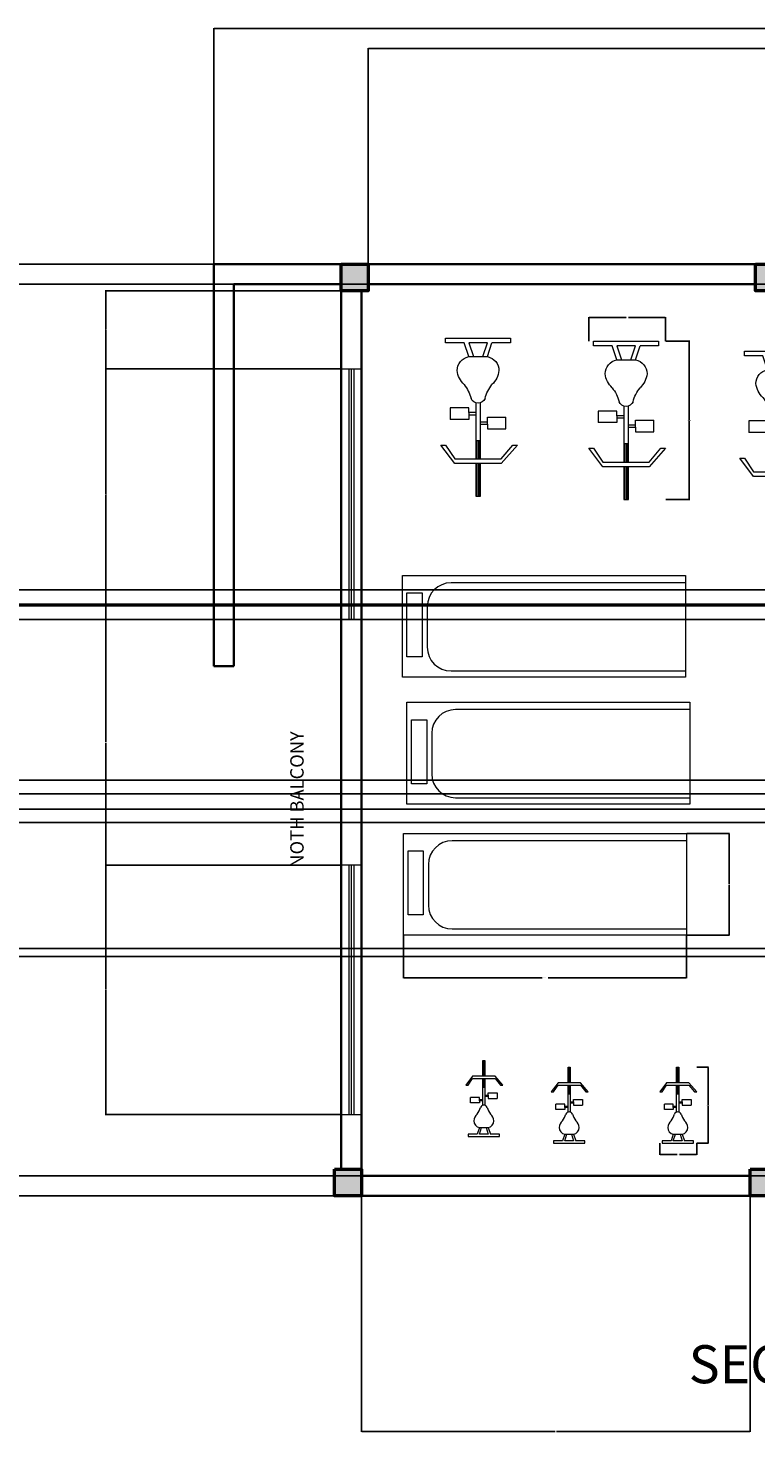
# Model space of a CAD drawing. Units: inches. Extents: x 369 to 4994, y 516 to 1297.
# Tile 7 of 9: x 1910 to 2235, y 516 to 1144. Entities that reach past the tile are written whole.
import ezdxf

# ---------------------------------------------------------------- set-up
doc = ezdxf.new("R2010")
doc.units = ezdxf.units.IN
doc.header["$MEASUREMENT"] = 0
for name, color, linetype, lineweight in [('A-ANNO-DIMS', 2, 'Continuous', 18), ('A-ANNO-TEXT', 7, 'Continuous', 35), ('A-AREA-IDEN', 7, 'Continuous', 18), ('A-COLS', 7, 'Continuous', 50), ('A-EQPM', 9, 'Continuous', 18), ('A-GLAZ', 4, 'Continuous', 18), ('A-WALL', 7, 'Continuous', 35)]:
    doc.layers.add(name, color=color, linetype=linetype, lineweight=lineweight)
doc.layers.add('A-COLS-PATT', color=18, linetype='Continuous', lineweight=13, true_color=0x000000)
doc.styles.get("Standard").update_dxf_attribs({"font": 'arial.ttf'})
doc.dimstyles.get("Standard").update_dxf_attribs({"dimtxt": 0.18, "dimasz": 0.18, "dimexe": 0.18, "dimexo": 0.0625, "dimgap": 0.09, "dimtad": 0, "dimtih": 1, "dimtoh": 1, "dimdec": 4, "dimzin": 0, "dimdsep": 46, "dimtxsty": 'Standard', "dimcen": 0.09, "dimadec": 0, "dimazin": 0, "dimtfac": 1, "dimtdec": 4, "dimtofl": 0, "dimtmove": 0, "dimatfit": 3, "dimfxl": 1, "dimtolj": 1, "dimtzin": 0, "dimarcsym": 0})

# ---------------------------------------------------------------- blocks, each defined once
blk = doc.blocks.new('Exercise Bike')
for p, q in [((-0.75, 10), (-0.75, 17)), ((-0.75, 17), (0.25, 17)), ((-0.5, 17), (-0.5, 9.9929)), ((-0.25, 10), (-0.25, 17)), ((0, 17), (0, 9.9929)), ((0.25, 17), (0.25, 10)), ((-5.25, 10), (-8.25, 6)), ((-0.75, 10), (-5.25, 10)), ((4.75, 10), (-0.75, 10)), ((8.25, 6), (4.75, 10)), ((-7.25, 6), (-5.25, 9)), ((-5.25, 9), (4.75, 9)), ((-0.75, 5), (-0.75, 9)), ((-0.5, 8.9396), (-0.5, 5)), ((-0.25, 5), (-0.25, 9)), ((0, 8.9396), (0, 5)), ((0.25, 9), (0.25, 5)), ((4.75, 9), (7.25, 6)), ((-8.25, 6), (-7.25, 6)), ((-0.75, -3.0635), (-0.75, 5)), ((-0.75, 5), (0.25, 5)), ((0.25, 5), (0.25, -3.0635)), ((7.25, 6), (8.25, 6)), ((-6.25, -2), (-6.25, 0.5)), ((-2.25, 0.5), (-6.25, 0.5)), ((-2.25, -0.5), (-2.25, 0.5)), ((0.25, 1.5), (1.75, 1.5)), ((0.25, 1), (1.75, 1)), ((1.75, 2.5), (5.75, 2.5)), ((1.75, 1.5), (1.75, 2.5)), ((1.75, 1.5), (1.75, 0)), ((1.75, 0), (5.75, 0)), ((5.75, 2.5), (5.75, 0)), ((-2.25, -2), (-6.25, -2)), ((-2.25, -0.5), (-0.75, -0.5)), ((-2.25, -1), (-2.25, -0.5)), ((-2.25, -1), (-2.25, -2)), ((-0.75, -1), (-2.25, -1)), ((-2.25, -13), (-3.25, -16)), ((-2.25, -16), (-1.25, -13)), ((-2.25, -13), (1.75, -13)), ((0.75, -13), (1.75, -16)), ((1.75, -13), (2.75, -16)), ((-7.25, -16), (-7.25, -17)), ((-4.75, -16), (-7.25, -16)), ((-7.25, -17), (6.75, -17)), ((-3.25, -16), (-4.75, -16)), ((1.75, -16), (-2.25, -16)), ((6.75, -16), (2.75, -16)), ((6.75, -17), (6.75, -16))]:
    blk.add_line(p, q)
for centre, radius, start, end in [((-0.25, -4.625), 1.625, 22.61987, 157.3801), ((-9.6692, -1.9154), 8.1889, 321.6175, 345.2525), ((9.1691, -1.9154), 8.1889, 194.7476, 218.3825), ((0.1685, -10.5843), 4.9531, 133.6443, 173.2256), ((-0.6686, -10.5843), 4.9531, 6.774486, 46.35562), ((-1.7006, -10.0005), 3.0494, 179.9906, 259.6205), ((1.2006, -10.0005), 3.0494, 280.3795, 0.009389)]:
    blk.add_arc(centre, radius, start, end)
blk = doc.blocks.new('GYM-TREADMILL')
for p, q in [((126.66, 42.28), (21.77, 42.28)), ((11.14, 31.65), (11.14, 13.47)), ((21.77, 2.84), (126.66, 2.84))]:
    blk.add_line(p, q)
for points in [[(0, 45.56), (126.66, 45.56), (126.66, 0), (0, 0)], [(2.08, 37.74), (8.86, 37.74), (8.86, 9.1), (2.08, 9.1)]]:
    blk.add_lwpolyline(points, close=True)
for centre, start, end in [((21.77, 31.65), 90, 180), ((21.77, 13.47), 180, 270)]:
    blk.add_arc(centre, 10.63, start, end)
blk = doc.blocks.new('BALCONY-EDGE')
for p, q in [((57, 180), (0, 180)), ((0, 180), (0, 0)), ((9, 171), (9, 0)), ((57, 171), (9, 171)), ((9, 0), (0, 0))]:
    blk.add_line(p, q)
blk = doc.blocks.new('*D31')
at = {"layer": 'A-ANNO-DIMS', "color": 0, "lineweight": -2, "transparency": 16777216}
for p, q in [((2209.04, 679.42), (2214.25, 679.42)), ((2214.07, 679.24), (2214.07, 662.61)), ((2214.07, 645.6), (2214.07, 662.24)), ((2209.04, 645.42), (2214.25, 645.42))]:
    blk.add_line(p, q, dxfattribs=at)
at = {"layer": 'A-ANNO-DIMS', "color": 0, "transparency": 16777216}
for points in [[(2214.04, 679.24), (2214.1, 679.24), (2214.07, 679.42)], [(2214.04, 645.6), (2214.1, 645.6), (2214.07, 645.42)]]:
    blk.add_solid(points, dxfattribs=at)
at = {"layer": 'Defpoints', "color": 0, "transparency": 16777216}
for p in [(2208.97, 679.42), (2214.07, 679.42), (2208.97, 645.42)]:
    blk.add_point(p, dxfattribs=at)
at = {"layer": 'A-ANNO-DIMS', "color": 0, "transparency": 16777216, "insert": (2214.07, 662.42), "char_height": 0.18, "attachment_point": 5}
blk.add_mtext('\\A1;BIKE 34 TYP.', dxfattribs=at)
blk = doc.blocks.new('*D32')
at = {"layer": 'A-ANNO-DIMS', "color": 0, "lineweight": -2, "transparency": 16777216}
for p, q in [((2192.47, 645.36), (2192.47, 640.14)), ((2208.97, 645.36), (2208.97, 640.14)), ((2192.65, 640.32), (2200.21, 640.32)), ((2208.79, 640.32), (2201.24, 640.32))]:
    blk.add_line(p, q, dxfattribs=at)
at = {"layer": 'A-ANNO-DIMS', "color": 0, "transparency": 16777216}
for points in [[(2192.65, 640.35), (2192.65, 640.29), (2192.47, 640.32)], [(2208.79, 640.35), (2208.79, 640.29), (2208.97, 640.32)]]:
    blk.add_solid(points, dxfattribs=at)
at = {"layer": 'Defpoints', "color": 0, "transparency": 16777216}
for p in [(2192.47, 645.42), (2208.97, 645.42), (2208.97, 640.32)]:
    blk.add_point(p, dxfattribs=at)
at = {"layer": 'A-ANNO-DIMS', "color": 0, "transparency": 16777216, "insert": (2200.72, 640.32), "char_height": 0.18, "attachment_point": 5}
blk.add_mtext('\\A1;17 TYP.', dxfattribs=at)
blk = doc.blocks.new('*D33')
at = {"layer": 'A-ANNO-DIMS', "color": 0, "lineweight": -2, "transparency": 16777216}
for p, q in [((2195.09, 1004.23), (2205.82, 1004.23)), ((2205.64, 1004.05), (2205.64, 969.04)), ((2205.64, 933.67), (2205.64, 968.68)), ((2195.09, 933.49), (2205.82, 933.49))]:
    blk.add_line(p, q, dxfattribs=at)
at = {"layer": 'A-ANNO-DIMS', "color": 0, "transparency": 16777216}
for points in [[(2205.61, 1004.05), (2205.67, 1004.05), (2205.64, 1004.23)], [(2205.61, 933.67), (2205.67, 933.67), (2205.64, 933.49)]]:
    blk.add_solid(points, dxfattribs=at)
at = {"layer": 'Defpoints', "color": 0, "transparency": 16777216}
for p in [(2195.03, 1004.23), (2195.03, 933.49), (2205.64, 933.49)]:
    blk.add_point(p, dxfattribs=at)
at = {"layer": 'A-ANNO-DIMS', "color": 0, "transparency": 16777216, "insert": (2205.64, 968.86), "char_height": 0.18, "attachment_point": 5}
blk.add_mtext('\\A1;BIKE 71 TYP.', dxfattribs=at)
blk = doc.blocks.new('*D34')
at = {"layer": 'A-ANNO-DIMS', "color": 0, "lineweight": -2, "transparency": 16777216}
for p, q in [((2160.71, 1004.29), (2160.71, 1015.02)), ((2160.89, 1014.84), (2177.34, 1014.84)), ((2194.85, 1014.84), (2178.4, 1014.84)), ((2195.03, 1004.29), (2195.03, 1015.02))]:
    blk.add_line(p, q, dxfattribs=at)
at = {"layer": 'A-ANNO-DIMS', "color": 0, "transparency": 16777216}
for points in [[(2160.89, 1014.87), (2160.89, 1014.81), (2160.71, 1014.84)], [(2194.85, 1014.87), (2194.85, 1014.81), (2195.03, 1014.84)]]:
    blk.add_solid(points, dxfattribs=at)
at = {"layer": 'Defpoints', "color": 0, "transparency": 16777216}
for p in [(2195.03, 1014.84), (2160.71, 1004.23), (2195.03, 1004.23)]:
    blk.add_point(p, dxfattribs=at)
at = {"layer": 'A-ANNO-DIMS', "color": 0, "transparency": 16777216, "insert": (2177.87, 1014.84), "char_height": 0.18, "attachment_point": 5}
blk.add_mtext('\\A1;34 TYP.', dxfattribs=at)
blk = doc.blocks.new('*D37')
at = {"layer": 'A-ANNO-DIMS', "color": 0, "lineweight": -2, "transparency": 16777216}
for p, q in [((2077.76, 738.39), (2077.76, 719.27)), ((2204.43, 738.39), (2204.43, 719.27)), ((2077.94, 719.45), (2139.75, 719.45)), ((2204.25, 719.45), (2142.44, 719.45))]:
    blk.add_line(p, q, dxfattribs=at)
at = {"layer": 'A-ANNO-DIMS', "color": 0, "transparency": 16777216}
for points in [[(2077.94, 719.48), (2077.94, 719.42), (2077.76, 719.45)], [(2204.25, 719.48), (2204.25, 719.42), (2204.43, 719.45)]]:
    blk.add_solid(points, dxfattribs=at)
at = {"layer": 'Defpoints', "color": 0, "transparency": 16777216}
for p in [(2077.76, 738.45), (2204.43, 738.45), (2204.43, 719.45)]:
    blk.add_point(p, dxfattribs=at)
at = {"layer": 'A-ANNO-DIMS', "color": 0, "transparency": 16777216, "insert": (2141.1, 719.45), "char_height": 0.18, "attachment_point": 5}
blk.add_mtext('\\A1;TREADMILL 127 TYP.', dxfattribs=at)
blk = doc.blocks.new('*D38')
at = {"layer": 'A-ANNO-DIMS', "color": 0, "lineweight": -2, "transparency": 16777216}
for p, q in [((2204.49, 784.01), (2223.6, 784.01)), ((2223.42, 783.83), (2223.42, 761.41)), ((2223.42, 738.63), (2223.42, 761.05)), ((2204.49, 738.45), (2223.6, 738.45))]:
    blk.add_line(p, q, dxfattribs=at)
at = {"layer": 'A-ANNO-DIMS', "color": 0, "transparency": 16777216}
for points in [[(2223.39, 783.83), (2223.45, 783.83), (2223.42, 784.01)], [(2223.39, 738.63), (2223.45, 738.63), (2223.42, 738.45)]]:
    blk.add_solid(points, dxfattribs=at)
at = {"layer": 'Defpoints', "color": 0, "transparency": 16777216}
for p in [(2204.43, 784.01), (2223.42, 784.01), (2204.43, 738.45)]:
    blk.add_point(p, dxfattribs=at)
at = {"layer": 'A-ANNO-DIMS', "color": 0, "transparency": 16777216, "insert": (2223.42, 761.23), "char_height": 0.18, "attachment_point": 5}
blk.add_mtext('\\A1;46 TYP.', dxfattribs=at)
blk = doc.blocks.new('*D46')
at = {"layer": 'A-ANNO-DIMS', "color": 0, "lineweight": -2, "transparency": 16777216}
for p, q in [((978.32, 1029.79), (2671.51, 1029.79)), ((2671.33, 1029.61), (2671.33, 957.97)), ((2671.33, 885.97), (2671.33, 957.61)), ((1038.32, 885.79), (2671.51, 885.79))]:
    blk.add_line(p, q, dxfattribs=at)
at = {"layer": 'A-ANNO-DIMS', "color": 0, "transparency": 16777216}
for points in [[(2671.3, 1029.61), (2671.36, 1029.61), (2671.33, 1029.79)], [(2671.3, 885.97), (2671.36, 885.97), (2671.33, 885.79)]]:
    blk.add_solid(points, dxfattribs=at)
at = {"layer": 'Defpoints', "color": 0, "transparency": 16777216}
for p in [(978.26, 1029.79), (2671.33, 1029.79), (1038.26, 885.79)]:
    blk.add_point(p, dxfattribs=at)
at = {"layer": 'A-ANNO-DIMS', "color": 0, "transparency": 16777216, "insert": (2671.33, 957.79), "char_height": 0.18, "attachment_point": 5}
blk.add_mtext('\\A1;144', dxfattribs=at)
blk = doc.blocks.new('*D47')
at = {"layer": 'A-ANNO-DIMS', "color": 0, "lineweight": -2, "transparency": 16777216}
for p, q in [((1038.32, 879.79), (2671.51, 879.79)), ((2671.33, 879.61), (2671.33, 837.52)), ((2671.33, 795.07), (2671.33, 837.16)), ((1035.32, 794.89), (2671.51, 794.89))]:
    blk.add_line(p, q, dxfattribs=at)
at = {"layer": 'A-ANNO-DIMS', "color": 0, "transparency": 16777216}
for points in [[(2671.3, 879.61), (2671.36, 879.61), (2671.33, 879.79)], [(2671.3, 795.07), (2671.36, 795.07), (2671.33, 794.89)]]:
    blk.add_solid(points, dxfattribs=at)
at = {"layer": 'Defpoints', "color": 0, "transparency": 16777216}
for p in [(1038.26, 879.79), (2671.33, 879.79), (1035.26, 794.89)]:
    blk.add_point(p, dxfattribs=at)
at = {"layer": 'A-ANNO-DIMS', "color": 0, "transparency": 16777216, "insert": (2671.33, 837.34), "char_height": 0.18, "attachment_point": 5}
blk.add_mtext('\\A1;84.9', dxfattribs=at)
blk = doc.blocks.new('*D52')
at = {"layer": 'A-ANNO-DIMS', "color": 0, "lineweight": -2, "transparency": 16777216}
for p, q in [((942.32, 788.89), (2671.51, 788.89)), ((2671.33, 788.71), (2671.33, 710.02)), ((2671.33, 630.97), (2671.33, 709.66)), ((1035.32, 630.79), (2671.51, 630.79))]:
    blk.add_line(p, q, dxfattribs=at)
at = {"layer": 'A-ANNO-DIMS', "color": 0, "transparency": 16777216}
for points in [[(2671.3, 788.71), (2671.36, 788.71), (2671.33, 788.89)], [(2671.3, 630.97), (2671.36, 630.97), (2671.33, 630.79)]]:
    blk.add_solid(points, dxfattribs=at)
at = {"layer": 'Defpoints', "color": 0, "transparency": 16777216}
for p in [(942.26, 788.89), (2671.33, 788.89), (1035.26, 630.79)]:
    blk.add_point(p, dxfattribs=at)
at = {"layer": 'A-ANNO-DIMS', "color": 0, "transparency": 16777216, "insert": (2671.33, 709.84), "char_height": 0.18, "attachment_point": 5}
blk.add_mtext('\\A1;158.1', dxfattribs=at)
blk = doc.blocks.new('*D79')
at = {"layer": 'A-ANNO-DIMS', "color": 0, "lineweight": -2, "transparency": 16777216}
for p, q in [((1769.44, 1029.79), (2671.51, 1029.79)), ((2671.33, 1029.61), (2671.33, 961.56)), ((2671.33, 893.15), (2671.33, 961.2)), ((1772.44, 892.97), (2671.51, 892.97))]:
    blk.add_line(p, q, dxfattribs=at)
at = {"layer": 'A-ANNO-DIMS', "color": 0, "transparency": 16777216}
for points in [[(2671.3, 1029.61), (2671.36, 1029.61), (2671.33, 1029.79)], [(2671.3, 893.15), (2671.36, 893.15), (2671.33, 892.97)]]:
    blk.add_solid(points, dxfattribs=at)
at = {"layer": 'Defpoints', "color": 0, "transparency": 16777216}
for p in [(1769.37, 1029.79), (2671.33, 1029.79), (1772.37, 892.97)]:
    blk.add_point(p, dxfattribs=at)
at = {"layer": 'A-ANNO-DIMS', "color": 0, "transparency": 16777216, "insert": (2671.33, 961.38), "char_height": 0.18, "attachment_point": 5}
blk.add_mtext('\\A1;136.82', dxfattribs=at)
blk = doc.blocks.new('*D80')
at = {"layer": 'A-ANNO-DIMS', "color": 0, "lineweight": -2, "transparency": 16777216}
for p, q in [((1772.44, 886.6), (2671.51, 886.6)), ((2671.33, 886.42), (2671.33, 847.38)), ((2671.33, 807.97), (2671.33, 847.01)), ((1772.44, 807.79), (2671.51, 807.79))]:
    blk.add_line(p, q, dxfattribs=at)
at = {"layer": 'A-ANNO-DIMS', "color": 0, "transparency": 16777216}
for points in [[(2671.3, 886.42), (2671.36, 886.42), (2671.33, 886.6)], [(2671.3, 807.97), (2671.36, 807.97), (2671.33, 807.79)]]:
    blk.add_solid(points, dxfattribs=at)
at = {"layer": 'Defpoints', "color": 0, "transparency": 16777216}
for p in [(1772.37, 886.6), (2671.33, 886.6), (1772.37, 807.79)]:
    blk.add_point(p, dxfattribs=at)
at = {"layer": 'A-ANNO-DIMS', "color": 0, "transparency": 16777216, "insert": (2671.33, 847.19), "char_height": 0.18, "attachment_point": 5}
blk.add_mtext('\\A1;78.81', dxfattribs=at)
blk = doc.blocks.new('*D85')
at = {"layer": 'A-ANNO-DIMS', "color": 0, "lineweight": -2, "transparency": 16777216}
for p, q in [((1772.44, 801.79), (2671.51, 801.79)), ((2671.33, 801.61), (2671.33, 767.36)), ((2671.33, 732.75), (2671.33, 767)), ((1772.44, 732.57), (2671.51, 732.57))]:
    blk.add_line(p, q, dxfattribs=at)
at = {"layer": 'A-ANNO-DIMS', "color": 0, "transparency": 16777216}
for points in [[(2671.3, 801.61), (2671.36, 801.61), (2671.33, 801.79)], [(2671.3, 732.75), (2671.36, 732.75), (2671.33, 732.57)]]:
    blk.add_solid(points, dxfattribs=at)
at = {"layer": 'Defpoints', "color": 0, "transparency": 16777216}
for p in [(1772.37, 801.79), (2671.33, 801.79), (1772.37, 732.57)]:
    blk.add_point(p, dxfattribs=at)
at = {"layer": 'A-ANNO-DIMS', "color": 0, "transparency": 16777216, "insert": (2671.33, 767.18), "char_height": 0.18, "attachment_point": 5}
blk.add_mtext('\\A1;69.22', dxfattribs=at)
blk = doc.blocks.new('*D86')
at = {"layer": 'A-ANNO-DIMS', "color": 0, "lineweight": -2, "transparency": 16777216}
for p, q in [((1772.44, 728.97), (2671.51, 728.97)), ((2671.33, 728.79), (2671.33, 680.06)), ((2671.33, 630.97), (2671.33, 679.7)), ((1769.44, 630.79), (2671.51, 630.79))]:
    blk.add_line(p, q, dxfattribs=at)
at = {"layer": 'A-ANNO-DIMS', "color": 0, "transparency": 16777216}
for points in [[(2671.3, 728.79), (2671.36, 728.79), (2671.33, 728.97)], [(2671.3, 630.97), (2671.36, 630.97), (2671.33, 630.79)]]:
    blk.add_solid(points, dxfattribs=at)
at = {"layer": 'Defpoints', "color": 0, "transparency": 16777216}
for p in [(1772.37, 728.97), (2671.33, 728.97), (1769.37, 630.79)]:
    blk.add_point(p, dxfattribs=at)
at = {"layer": 'A-ANNO-DIMS', "color": 0, "transparency": 16777216, "insert": (2671.33, 679.88), "char_height": 0.18, "attachment_point": 5}
blk.add_mtext('\\A1;98.18', dxfattribs=at)
blk = doc.blocks.new('*D97')
at = {"layer": 'A-ANNO-DIMS', "color": 0, "lineweight": -2, "transparency": 16777216}
for p, q in [((1992.93, 1038.85), (1992.93, 1144.37)), ((1993.11, 1144.19), (2279.14, 1144.19)), ((2565.75, 1144.19), (2279.72, 1144.19)), ((2565.93, 1038.85), (2565.93, 1144.37))]:
    blk.add_line(p, q, dxfattribs=at)
at = {"layer": 'A-ANNO-DIMS', "color": 0, "transparency": 16777216}
for points in [[(1993.11, 1144.22), (1993.11, 1144.16), (1992.93, 1144.19)], [(2565.75, 1144.22), (2565.75, 1144.16), (2565.93, 1144.19)]]:
    blk.add_solid(points, dxfattribs=at)
at = {"layer": 'Defpoints', "color": 0, "transparency": 16777216}
for p in [(2565.93, 1144.19), (1992.93, 1038.79), (2565.93, 1038.79)]:
    blk.add_point(p, dxfattribs=at)
at = {"layer": 'A-ANNO-DIMS', "color": 0, "transparency": 16777216, "insert": (2279.43, 1144.19), "char_height": 0.18, "attachment_point": 5}
blk.add_mtext('\\A1;573', dxfattribs=at)
blk = doc.blocks.new('*D98')
at = {"layer": 'A-ANNO-DIMS', "color": 0, "lineweight": -2, "transparency": 16777216}
for p, q in [((1992.86, 1038.79), (368.68, 1038.79)), ((368.86, 1038.61), (368.86, 830.47)), ((368.86, 621.97), (368.86, 830.11)), ((2046.86, 621.79), (368.68, 621.79))]:
    blk.add_line(p, q, dxfattribs=at)
at = {"layer": 'A-ANNO-DIMS', "color": 0, "transparency": 16777216}
for points in [[(368.83, 1038.61), (368.89, 1038.61), (368.86, 1038.79)], [(368.83, 621.97), (368.89, 621.97), (368.86, 621.79)]]:
    blk.add_solid(points, dxfattribs=at)
at = {"layer": 'Defpoints', "color": 0, "transparency": 16777216}
for p in [(368.86, 1038.79), (1992.93, 1038.79), (2046.93, 621.79)]:
    blk.add_point(p, dxfattribs=at)
at = {"layer": 'A-ANNO-DIMS', "color": 0, "transparency": 16777216, "insert": (368.86, 830.29), "char_height": 0.18, "attachment_point": 5}
blk.add_mtext('\\A1;417', dxfattribs=at)
blk = doc.blocks.new('*D99')
at = {"layer": 'A-ANNO-DIMS', "color": 0, "lineweight": -2, "transparency": 16777216}
for p, q in [((2061.93, 1029.85), (2061.93, 1135.37)), ((2062.11, 1135.19), (2241.64, 1135.19)), ((2421.75, 1135.19), (2242.22, 1135.19)), ((2421.93, 1029.85), (2421.93, 1135.37))]:
    blk.add_line(p, q, dxfattribs=at)
at = {"layer": 'A-ANNO-DIMS', "color": 0, "transparency": 16777216}
for points in [[(2062.11, 1135.22), (2062.11, 1135.16), (2061.93, 1135.19)], [(2421.75, 1135.22), (2421.75, 1135.16), (2421.93, 1135.19)]]:
    blk.add_solid(points, dxfattribs=at)
at = {"layer": 'Defpoints', "color": 0, "transparency": 16777216}
for p in [(2421.93, 1135.19), (2061.93, 1029.79), (2421.93, 1029.79)]:
    blk.add_point(p, dxfattribs=at)
at = {"layer": 'A-ANNO-DIMS', "color": 0, "transparency": 16777216, "insert": (2241.93, 1135.19), "char_height": 0.18, "attachment_point": 5}
blk.add_mtext('\\A1;360', dxfattribs=at)
blk = doc.blocks.new('*D108')
at = {"layer": 'A-ANNO-DIMS', "color": 0, "lineweight": -2, "transparency": 16777216}
for p, q in [((2058.93, 630.73), (2058.93, 516.21)), ((2232.93, 630.73), (2232.93, 516.21)), ((2059.11, 516.39), (2145.65, 516.39)), ((2232.75, 516.39), (2146.21, 516.39))]:
    blk.add_line(p, q, dxfattribs=at)
at = {"layer": 'A-ANNO-DIMS', "color": 0, "transparency": 16777216}
for points in [[(2059.11, 516.42), (2059.11, 516.36), (2058.93, 516.39)], [(2232.75, 516.42), (2232.75, 516.36), (2232.93, 516.39)]]:
    blk.add_solid(points, dxfattribs=at)
at = {"layer": 'Defpoints', "color": 0, "transparency": 16777216}
for p in [(2058.93, 630.79), (2232.93, 630.79), (2232.93, 516.39)]:
    blk.add_point(p, dxfattribs=at)
at = {"layer": 'A-ANNO-DIMS', "color": 0, "transparency": 16777216, "insert": (2145.93, 516.39), "char_height": 0.18, "attachment_point": 5}
blk.add_mtext('\\A1;174', dxfattribs=at)
blk = doc.blocks.new('*D112')
at = {"layer": 'A-ANNO-DIMS', "color": 0, "lineweight": -2, "transparency": 16777216}
for p, q in [((2049.86, 1026.79), (1944.35, 1026.79)), ((1944.53, 1026.61), (1944.53, 1009.52)), ((1944.53, 992.06), (1944.53, 1009.15)), ((2049.86, 991.88), (1944.35, 991.88))]:
    blk.add_line(p, q, dxfattribs=at)
at = {"layer": 'A-ANNO-DIMS', "color": 0, "transparency": 16777216}
for points in [[(1944.5, 1026.61), (1944.56, 1026.61), (1944.53, 1026.79)], [(1944.5, 992.06), (1944.56, 992.06), (1944.53, 991.88)]]:
    blk.add_solid(points, dxfattribs=at)
at = {"layer": 'Defpoints', "color": 0, "transparency": 16777216}
for p in [(1944.53, 1026.79), (2049.93, 1026.79), (2049.93, 991.88)]:
    blk.add_point(p, dxfattribs=at)
at = {"layer": 'A-ANNO-DIMS', "color": 0, "transparency": 16777216, "insert": (1944.53, 1009.33), "char_height": 0.18, "attachment_point": 5}
blk.add_mtext('\\A1;34.91', dxfattribs=at)
blk = doc.blocks.new('*D113')
at = {"layer": 'A-ANNO-DIMS', "color": 0, "lineweight": -2, "transparency": 16777216}
for p, q in [((2049.86, 991.88), (1944.35, 991.88)), ((1944.53, 991.7), (1944.53, 936.02)), ((1944.53, 879.97), (1944.53, 935.65)), ((2049.86, 879.79), (1944.35, 879.79))]:
    blk.add_line(p, q, dxfattribs=at)
at = {"layer": 'A-ANNO-DIMS', "color": 0, "transparency": 16777216}
for points in [[(1944.5, 991.7), (1944.56, 991.7), (1944.53, 991.88)], [(1944.5, 879.97), (1944.56, 879.97), (1944.53, 879.79)]]:
    blk.add_solid(points, dxfattribs=at)
at = {"layer": 'Defpoints', "color": 0, "transparency": 16777216}
for p in [(1944.53, 991.88), (2049.93, 991.88), (2049.93, 879.79)]:
    blk.add_point(p, dxfattribs=at)
at = {"layer": 'A-ANNO-DIMS', "color": 0, "transparency": 16777216, "insert": (1944.53, 935.83), "char_height": 0.18, "attachment_point": 5}
blk.add_mtext('\\A1;112.09', dxfattribs=at)
blk = doc.blocks.new('*D114')
at = {"layer": 'A-ANNO-DIMS', "color": 0, "lineweight": -2, "transparency": 16777216}
for p, q in [((2049.86, 879.79), (1944.35, 879.79)), ((1944.53, 879.61), (1944.53, 824.97)), ((1944.53, 769.97), (1944.53, 824.61)), ((2049.86, 769.79), (1944.35, 769.79))]:
    blk.add_line(p, q, dxfattribs=at)
at = {"layer": 'A-ANNO-DIMS', "color": 0, "transparency": 16777216}
for points in [[(1944.5, 879.61), (1944.56, 879.61), (1944.53, 879.79)], [(1944.5, 769.97), (1944.56, 769.97), (1944.53, 769.79)]]:
    blk.add_solid(points, dxfattribs=at)
at = {"layer": 'Defpoints', "color": 0, "transparency": 16777216}
for p in [(1944.53, 879.79), (2049.93, 879.79), (2049.93, 769.79)]:
    blk.add_point(p, dxfattribs=at)
at = {"layer": 'A-ANNO-DIMS', "color": 0, "transparency": 16777216, "insert": (1944.53, 824.79), "char_height": 0.18, "attachment_point": 5}
blk.add_mtext('\\A1;110', dxfattribs=at)
blk = doc.blocks.new('*D115')
at = {"layer": 'A-ANNO-DIMS', "color": 0, "lineweight": -2, "transparency": 16777216}
for p, q in [((2049.86, 769.79), (1944.35, 769.79)), ((1944.53, 769.61), (1944.53, 714.2)), ((1944.53, 658.42), (1944.53, 713.84)), ((2049.86, 658.24), (1944.35, 658.24))]:
    blk.add_line(p, q, dxfattribs=at)
at = {"layer": 'A-ANNO-DIMS', "color": 0, "transparency": 16777216}
for points in [[(1944.5, 769.61), (1944.56, 769.61), (1944.53, 769.79)], [(1944.5, 658.42), (1944.56, 658.42), (1944.53, 658.24)]]:
    blk.add_solid(points, dxfattribs=at)
at = {"layer": 'Defpoints', "color": 0, "transparency": 16777216}
for p in [(1944.53, 769.79), (2049.93, 769.79), (2049.93, 658.24)]:
    blk.add_point(p, dxfattribs=at)
at = {"layer": 'A-ANNO-DIMS', "color": 0, "transparency": 16777216, "insert": (1944.53, 714.02), "char_height": 0.18, "attachment_point": 5}
blk.add_mtext('\\A1;111.55', dxfattribs=at)

msp = doc.modelspace()

# ---------------------------------------------------------------- hatches: boundary and pattern name
at = {"layer": 'A-COLS-PATT'}
h = msp.add_hatch(color=256, dxfattribs=at)
h.dxf.hatch_style = 1
h.paths.add_polyline_path([(540.2581, 633.7894), (528.2581, 633.7894), (528.2581, 621.7894), (540.2581, 621.7894)])
h.paths.add_polyline_path([(726.2581, 633.7894), (714.2581, 633.7894), (714.2581, 621.7894), (726.2581, 621.7894)])
h.paths.add_polyline_path([(918.2581, 633.7894), (906.2581, 633.7894), (906.2581, 621.7894), (918.2581, 621.7894)])
h.paths.add_polyline_path([(1047.2581, 633.7894), (1035.2581, 633.7894), (1035.2581, 621.7894), (1047.2581, 621.7894)])
h.paths.add_polyline_path([(1047.2581, 798.6977), (1035.2581, 798.6977), (1035.2581, 786.6977), (1047.2581, 786.6977)])
h.paths.add_polyline_path([(918.2581, 795.7894), (906.2581, 795.7894), (906.2581, 783.7894), (918.2581, 783.7894)])
h.paths.add_polyline_path([(726.2581, 795.7894), (714.2581, 795.7894), (714.2581, 783.7894), (726.2581, 783.7894)])
h.paths.add_polyline_path([(1047.2581, 1038.7894), (1035.2581, 1038.7894), (1035.2581, 1026.7894), (1047.2581, 1026.7894)])
h.paths.add_polyline_path([(855.044, 1038.7894), (843.044, 1038.7894), (843.044, 1026.7894), (855.044, 1026.7894)])
h.paths.add_polyline_path([(728.5536, 1038.7894), (716.5536, 1038.7894), (716.5536, 1026.7894), (728.5536, 1026.7894)])
h.paths.add_polyline_path([(543.2581, 1038.7894), (531.2581, 1038.7894), (531.2581, 1026.7894), (543.2581, 1026.7894)])
h.paths.add_polyline_path([(543.2581, 792.9013), (531.2581, 792.9013), (531.2581, 780.9013), (543.2581, 780.9013), (543.2581, 783.7894)])
h.paths.add_polyline_path([(1274.3738, 633.7894), (1262.3738, 633.7894), (1262.3738, 621.7894), (1274.3738, 621.7894)])
h.paths.add_polyline_path([(1460.3738, 633.7894), (1448.3738, 633.7894), (1448.3738, 621.7894), (1460.3738, 621.7894)])
h.paths.add_polyline_path([(1652.3738, 633.7894), (1640.3738, 633.7894), (1640.3738, 621.7894), (1652.3738, 621.7894)])
h.paths.add_polyline_path([(1781.3738, 633.7894), (1769.3738, 633.7894), (1769.3738, 621.7894), (1781.3738, 621.7894)])
h.paths.add_polyline_path([(1781.3738, 1038.7894), (1769.3738, 1038.7894), (1769.3738, 1026.7894), (1781.3738, 1026.7894)])
h.paths.add_polyline_path([(1625.484, 1038.7894), (1613.484, 1038.7894), (1613.484, 1026.7894), (1615.6962, 1026.7894), (1625.484, 1026.7894)])
h.paths.add_polyline_path([(1462.6692, 1038.7894), (1450.6692, 1038.7894), (1450.6692, 1026.7894), (1462.6692, 1026.7894)])
h.paths.add_polyline_path([(1277.3738, 1038.7894), (1265.3738, 1038.7894), (1265.3738, 1026.7894), (1277.3738, 1026.7894)])
h.paths.add_polyline_path([(1460.3738, 807.7894), (1448.3738, 807.7894), (1448.3738, 795.7894), (1460.3738, 795.7894)])
h.paths.add_polyline_path([(1652.3738, 807.7894), (1640.3738, 807.7894), (1640.3738, 795.7894), (1652.3738, 795.7894)])
h.paths.add_polyline_path([(2244.9265, 633.7894), (2232.9265, 633.7894), (2232.9265, 621.7894), (2244.9265, 621.7894)])
h.paths.add_polyline_path([(2058.9265, 633.7894), (2046.9265, 633.7894), (2046.9265, 621.7894), (2058.9265, 621.7894)])
h.paths.add_polyline_path([(2436.9265, 633.7894), (2424.9265, 633.7894), (2424.9265, 621.7894), (2436.9265, 621.7894)])
h.paths.add_polyline_path([(2565.9265, 633.7894), (2553.9265, 633.7894), (2553.9265, 621.7894), (2565.9265, 621.7894)])
h.paths.add_polyline_path([(2565.9265, 798.6977), (2553.9265, 798.6977), (2553.9265, 786.6977), (2565.9265, 786.6977)])
h.paths.add_polyline_path([(2565.9265, 1038.7894), (2553.9265, 1038.7894), (2553.9265, 1026.7894), (2565.9265, 1026.7894)])
h.paths.add_polyline_path([(2436.9265, 1038.7894), (2424.9265, 1038.7894), (2424.9265, 1026.7894), (2436.9265, 1026.7894)])
h.paths.add_polyline_path([(2247.222, 1038.7894), (2235.222, 1038.7894), (2235.222, 1026.7894), (2247.222, 1026.7894)])
h.paths.add_polyline_path([(2061.9265, 1038.7894), (2049.9265, 1038.7894), (2049.9265, 1026.7894), (2061.9265, 1026.7894)])

# ---------------------------------------------------------------- linework, layer by layer
at = {"layer": 'A-COLS'}
for points in [[(2049.9265, 1038.7894), (2061.9265, 1038.7894), (2061.9265, 1026.7894), (2049.9265, 1026.7894)], [(2235.222, 1038.7894), (2247.222, 1038.7894), (2247.222, 1026.7894), (2235.222, 1026.7894)], [(2046.9265, 633.7894), (2058.9265, 633.7894), (2058.9265, 621.7894), (2046.9265, 621.7894)], [(2232.9265, 633.7894), (2244.9265, 633.7894), (2244.9265, 621.7894), (2232.9265, 621.7894)]]:
    msp.add_lwpolyline(points, close=True, dxfattribs=at)
at = {"layer": 'A-EQPM'}
msp.add_line((2205.9457, 839.4483), (2205.9457, 839.4483), dxfattribs=at)
at = {"layer": 'A-GLAZ'}
for p, q in [((2053.3504, 991.8774), (2053.3504, 879.7894)), ((2054.4265, 991.8774), (2054.4265, 879.7894)), ((2055.5026, 991.8774), (2055.5026, 879.7894)), ((2053.3504, 769.7944), (2053.3504, 658.2425)), ((2054.4265, 769.7944), (2054.4265, 658.2425)), ((2055.5026, 769.7944), (2055.5026, 658.2425))]:
    msp.add_line(p, q, dxfattribs=at)
for points in [[(2049.9265, 991.8774), (2058.9265, 991.8774), (2058.9265, 879.7894), (2049.9265, 879.7894)], [(2058.9265, 769.7944), (2049.9265, 769.7944), (2049.9265, 658.2425), (2058.9265, 658.2425)]]:
    msp.add_lwpolyline(points, close=True, dxfattribs=at)
at = {"layer": 'A-WALL'}
for p, q in [((2556.9265, 1038.7894), (2049.9265, 1038.7894)), ((2049.9265, 1029.7894), (2049.9265, 633.7894)), ((2058.9265, 792.9013), (2058.9265, 1026.7894)), ((2235.222, 1029.7894), (2061.9265, 1029.7894)), ((2184.9265, 1029.7894), (2061.9265, 1029.7894)), ((2058.9265, 792.9013), (2058.9265, 879.7894)), ((2058.9265, 792.9013), (2058.9265, 849.7894)), ((2058.9265, 780.9013), (2058.9265, 792.9013)), ((2058.9265, 780.9013), (2058.9265, 633.7894)), ((2058.9265, 630.7894), (2178.9265, 630.7894)), ((2058.9265, 630.7894), (2232.9265, 630.7894)), ((2058.9265, 621.7894), (2178.9265, 621.7894)), ((2178.9265, 621.7894), (2232.9265, 621.7894))]:
    msp.add_line(p, q, dxfattribs=at)

# ---------------------------------------------------------------- block references
at = {"layer": 'A-EQPM', "xscale": -2.080401215836593, "yscale": 2.080401215836593, "zscale": 2.080401215836593, "rotation": 180}
for p in [(2111.6442, 970.2954), (2177.8688, 968.8583), (2245.3378, 964.4622)]:
    msp.add_blockref('Exercise Bike', p, dxfattribs=at)
at = {"layer": 'A-EQPM'}
for name, p in [('GYM-TREADMILL', (2077.258, 853.864)), ('GYM-TREADMILL', (2079.2846, 797.1685)), ('GYM-TREADMILL', (2077.7647, 738.4482)), ('Exercise Bike', (2113.9642, 665.4234)), ('Exercise Bike', (2152.1444, 662.4234)), ('Exercise Bike', (2200.725, 662.4234))]:
    msp.add_blockref(name, p, dxfattribs=at)
at = {"layer": 'A-WALL'}
msp.add_blockref('BALCONY-EDGE', (1992.9264, 858.789), dxfattribs=at)

# ---------------------------------------------------------------- texts
at = {"layer": 'A-ANNO-TEXT'}
msp.add_text('SECOND FLOOR', height=17.017766, dxfattribs=at).set_placement((2205.3764, 537.9843))
at = {"layer": 'A-AREA-IDEN'}
msp.add_text('NOTH BALCONY ', height=6, rotation=90, dxfattribs=at).set_placement((2033.1012, 768.6802))

# ---------------------------------------------------------------- dimensions: what is measured, and where the dimension line sits
at = {"layer": 'A-ANNO-DIMS'}
for base, p1, p2, picture, middle in [((2565.9265, 1144.1894), (1992.9265, 1038.7894), (2565.9265, 1038.7894), '*D97', (2279.4265, 1144.1894)), ((2421.9265, 1135.1894), (2061.9265, 1029.7894), (2421.9265, 1029.7894), '*D99', (2241.9265, 1135.1894)), ((2232.9265, 516.3894), (2058.9265, 630.7894), (2232.9265, 630.7894), '*D108', (2145.9265, 516.3894))]:
    dim = msp.add_linear_dim(base=base, p1=p1, p2=p2, dimstyle='Standard', override={"dimdec": 0, "dimlfac": 1, "dimrnd": 0, "dimzin": 0, "dimdsep": 46, "dimlunit": 2}, dxfattribs=at)
    dim.commit()
    dim.dimension.update_dxf_attribs({"geometry": picture, "text_midpoint": middle})
for base, p1, p2, override, picture, middle in [((368.8581, 1038.7894), (2046.9265, 621.7894), (1992.9265, 1038.7894), {"dimdec": 0, "dimlfac": 1, "dimrnd": 0, "dimzin": 0, "dimdsep": 46, "dimlunit": 2}, '*D98', (368.8581, 830.2894)), ((2671.3265, 1029.7894), (1038.2581, 885.7894), (978.2581, 1029.7894), {"dimdec": 0, "dimlfac": 1, "dimrnd": 0, "dimzin": 0, "dimdsep": 46, "dimlunit": 2}, '*D46', (2671.3265, 957.7894)), ((2671.3265, 1029.7894), (1772.3738, 892.9667), (1769.3738, 1029.7894), {"dimdec": 2, "dimlfac": 1, "dimrnd": 0, "dimzin": 0, "dimdsep": 46, "dimlunit": 2}, '*D79', (2671.3265, 961.378)), ((1944.5265, 1026.7894), (2049.9265, 991.8774), (2049.9265, 1026.7894), {"dimdec": 2, "dimlfac": 1, "dimrnd": 0, "dimzin": 0, "dimdsep": 46, "dimlunit": 2}, '*D112', (1944.5265, 1009.3334)), ((1944.5265, 991.8774), (2049.9265, 879.7894), (2049.9265, 991.8774), {"dimdec": 2, "dimlfac": 1, "dimrnd": 0, "dimzin": 0, "dimdsep": 46, "dimlunit": 2}, '*D113', (1944.5265, 935.8334)), ((2671.3265, 886.5988), (1772.3738, 807.7894), (1772.3738, 886.5988), {"dimdec": 2, "dimlfac": 1, "dimrnd": 0, "dimzin": 0, "dimdsep": 46, "dimlunit": 2}, '*D80', (2671.3265, 847.1941)), ((2671.3265, 879.7894), (1035.2581, 794.8925), (1038.2581, 879.7894), {"dimdec": 1, "dimlfac": 1, "dimrnd": 0, "dimzin": 0, "dimdsep": 46, "dimlunit": 2}, '*D47', (2671.3265, 837.3409)), ((1944.5265, 879.7894), (2049.9265, 769.7944), (2049.9265, 879.7894), {"dimdec": 0, "dimlfac": 1, "dimrnd": 0, "dimzin": 0, "dimdsep": 46, "dimlunit": 2}, '*D114', (1944.5265, 824.7919)), ((2671.3265, 801.7894), (1772.3738, 732.5675), (1772.3738, 801.7894), {"dimdec": 2, "dimlfac": 1, "dimrnd": 0, "dimzin": 0, "dimdsep": 46, "dimlunit": 2}, '*D85', (2671.3265, 767.1784)), ((2671.3265, 788.8925), (1035.2581, 630.7894), (942.2581, 788.8925), {"dimdec": 1, "dimlfac": 1, "dimrnd": 0, "dimzin": 0, "dimdsep": 46, "dimlunit": 2}, '*D52', (2671.3265, 709.8409)), ((1944.5265, 769.7944), (2049.9265, 658.2425), (2049.9265, 769.7944), {"dimdec": 2, "dimlfac": 1, "dimrnd": 0, "dimzin": 0, "dimdsep": 46, "dimlunit": 2}, '*D115', (1944.5265, 714.0185)), ((2671.3265, 728.9712), (1769.3738, 630.7894), (1772.3738, 728.9712), {"dimdec": 2, "dimlfac": 1, "dimrnd": 0, "dimzin": 0, "dimdsep": 46, "dimlunit": 2}, '*D86', (2671.3265, 679.8803))]:
    dim = msp.add_linear_dim(base=base, p1=p1, p2=p2, angle=90, dimstyle='Standard', override=override, dxfattribs=at)
    dim.commit()
    dim.dimension.update_dxf_attribs({"geometry": picture, "text_midpoint": middle})
for base, p1, p2, text, picture, middle in [((2195.0321, 1014.8352), (2160.7055, 1004.2251), (2195.0321, 1004.2251), '<> TYP.', '*D34', (2177.8688, 1014.8352)), ((2204.4257, 719.4492), (2077.7644, 738.4484), (2204.4257, 738.4484), 'TREADMILL <> TYP.', '*D37', (2141.0951, 719.4492)), ((2208.97498833, 640.3233982265), (2192.47498833, 645.4233982265), (2208.97498833, 645.4233982265), '<> TYP.', '*D32', (2200.72498833, 640.3233982265))]:
    dim = msp.add_linear_dim(base=base, p1=p1, p2=p2, text=text, dimstyle='Standard', override={"dimdec": 0, "dimlfac": 1, "dimrnd": 0, "dimzin": 0, "dimdsep": 46, "dimlunit": 2}, dxfattribs=at)
    dim.commit()
    dim.dimension.update_dxf_attribs({"geometry": picture, "text_midpoint": middle})
for base, p1, p2, angle, text, picture, middle in [((2205.6422, 933.4915), (2195.0321, 1004.2251), (2195.0321, 933.4915), 270, 'BIKE <> TYP.', '*D33', (2205.6422, 968.8583)), ((2223.4249, 784.0073), (2204.4257, 738.4484), (2204.4257, 784.0073), 90, '<> TYP.', '*D38', (2223.4249, 761.2279)), ((2214.075, 679.4234), (2208.975, 645.4234), (2208.975, 679.4234), 90, 'BIKE <> TYP.', '*D31', (2214.075, 662.4234))]:
    dim = msp.add_linear_dim(base=base, p1=p1, p2=p2, angle=angle, text=text, dimstyle='Standard', override={"dimdec": 0, "dimlfac": 1, "dimrnd": 0, "dimzin": 0, "dimdsep": 46, "dimlunit": 2}, dxfattribs=at)
    dim.commit()
    dim.dimension.update_dxf_attribs({"geometry": picture, "text_midpoint": middle})

doc.saveas('drawing.dxf')
